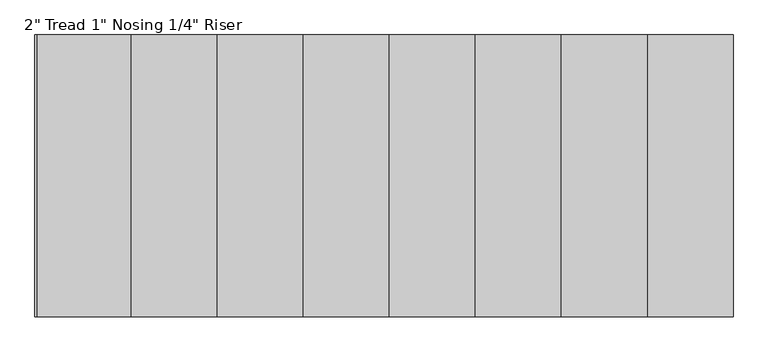
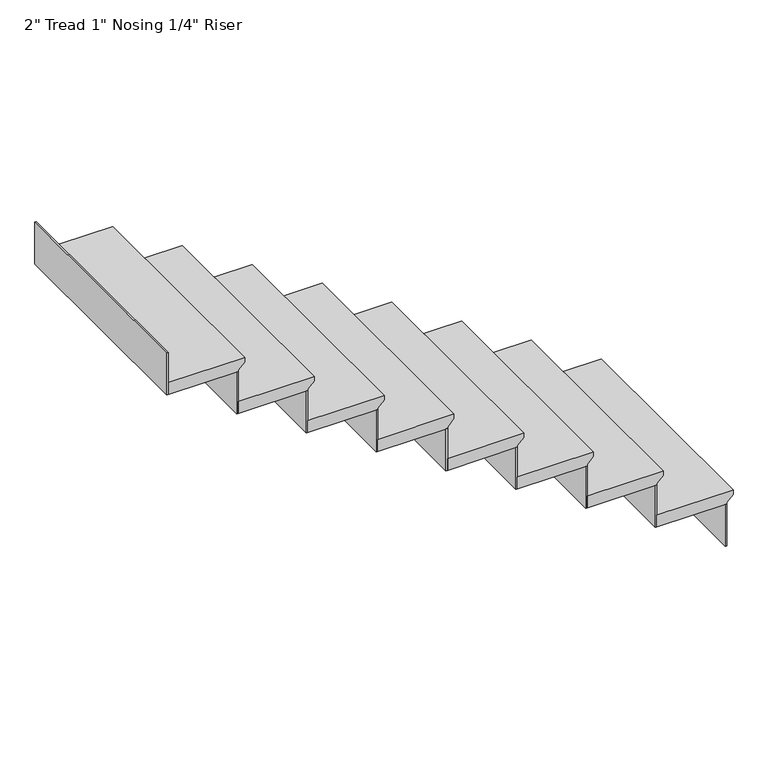
"""IFC4 building model written with IfcOpenShell, lengths in millimetres: stair flight geometry."""

from ifc_helpers import new_model, si_unit, frame, origin, place, context, project, spatial, polyline, outline, extrude, source, transform, mapped, element, save


def stair_flight_9d7122d5(model_context):
    return source(origin(), model_context, "Body", "SweptSolid", [
        extrude(outline(polyline([(1778.0, -2178.613859), (1778.0, -2483.413859), (1727.2, -2483.413859), (1727.2, -2204.013859), (1733.55, -2204.013859), (1758.95, -2178.613859), (1778.0, -2178.613859)])), frame((0.0, -712.1793133, 0.0), z_axis=(0.0, 1.0, 0.0), x_axis=(0.0, 0.0, 1.0)), (0.0, 0.0, 1.0), 914.4),
        extrude(outline(polyline([(-2210.363859, 202.2206867), (-2204.013859, 202.2206867), (-2204.013859, -712.1793133), (-2210.363859, -712.1793133), (-2210.363859, 202.2206867)])), frame((0.0, 0.0, 1549.4), z_axis=(0.0, 0.0, 1.0), x_axis=(1.0, 0.0, 0.0)), (0.0, 0.0, 1.0), 177.8),
        extrude(outline(polyline([(-2489.763859, 202.2206867), (-2483.413859, 202.2206867), (-2483.413859, -712.1793133), (-2489.763859, -712.1793133), (-2489.763859, 202.2206867)])), frame((0.0, 0.0, 1727.2), z_axis=(0.0, 0.0, 1.0), x_axis=(1.0, 0.0, 0.0)), (0.0, 0.0, 1.0), 177.8),
        extrude(outline(polyline([(1955.8, -2458.013859), (1955.8, -2762.813859), (1905.0, -2762.813859), (1905.0, -2483.413859), (1911.35, -2483.413859), (1936.75, -2458.013859), (1955.8, -2458.013859)])), frame((0.0, -712.1793133, 0.0), z_axis=(0.0, 1.0, 0.0), x_axis=(0.0, 0.0, 1.0)), (0.0, 0.0, 1.0), 914.4),
        extrude(outline(polyline([(-2769.163859, 202.2206867), (-2762.813859, 202.2206867), (-2762.813859, -712.1793133), (-2769.163859, -712.1793133), (-2769.163859, 202.2206867)])), frame((0.0, 0.0, 1905.0), z_axis=(0.0, 0.0, 1.0), x_axis=(1.0, 0.0, 0.0)), (0.0, 0.0, 1.0), 177.8),
        extrude(outline(polyline([(2133.6, -2737.413859), (2133.6, -3042.213859), (2082.8, -3042.213859), (2082.8, -2762.813859), (2089.15, -2762.813859), (2114.55, -2737.413859), (2133.6, -2737.413859)])), frame((0.0, -712.1793133, 0.0), z_axis=(0.0, 1.0, 0.0), x_axis=(0.0, 0.0, 1.0)), (0.0, 0.0, 1.0), 914.4),
        extrude(outline(polyline([(-3048.563859, 202.2206867), (-3042.213859, 202.2206867), (-3042.213859, -712.1793133), (-3048.563859, -712.1793133), (-3048.563859, 202.2206867)])), frame((0.0, 0.0, 2082.8), z_axis=(0.0, 0.0, 1.0), x_axis=(1.0, 0.0, 0.0)), (0.0, 0.0, 1.0), 177.8),
        extrude(outline(polyline([(2311.4, -3016.813859), (2311.4, -3321.613859), (2260.6, -3321.613859), (2260.6, -3042.213859), (2266.95, -3042.213859), (2292.35, -3016.813859), (2311.4, -3016.813859)])), frame((0.0, -712.1793133, 0.0), z_axis=(0.0, 1.0, 0.0), x_axis=(0.0, 0.0, 1.0)), (0.0, 0.0, 1.0), 914.4),
        extrude(outline(polyline([(-3327.963859, 202.2206867), (-3321.613859, 202.2206867), (-3321.613859, -712.1793133), (-3327.963859, -712.1793133), (-3327.963859, 202.2206867)])), frame((0.0, 0.0, 2260.6), z_axis=(0.0, 0.0, 1.0), x_axis=(1.0, 0.0, 0.0)), (0.0, 0.0, 1.0), 177.8),
        extrude(outline(polyline([(2489.2, -3296.213859), (2489.2, -3601.013859), (2438.4, -3601.013859), (2438.4, -3321.613859), (2444.75, -3321.613859), (2470.15, -3296.213859), (2489.2, -3296.213859)])), frame((0.0, -712.1793133, 0.0), z_axis=(0.0, 1.0, 0.0), x_axis=(0.0, 0.0, 1.0)), (0.0, 0.0, 1.0), 914.4),
        extrude(outline(polyline([(-3607.363859, 202.2206867), (-3601.013859, 202.2206867), (-3601.013859, -712.1793133), (-3607.363859, -712.1793133), (-3607.363859, 202.2206867)])), frame((0.0, 0.0, 2438.4), z_axis=(0.0, 0.0, 1.0), x_axis=(1.0, 0.0, 0.0)), (0.0, 0.0, 1.0), 177.8),
        extrude(outline(polyline([(2667.0, -3575.613859), (2667.0, -3880.413859), (2616.2, -3880.413859), (2616.2, -3601.013859), (2622.55, -3601.013859), (2647.95, -3575.613859), (2667.0, -3575.613859)])), frame((0.0, -712.1793133, 0.0), z_axis=(0.0, 1.0, 0.0), x_axis=(0.0, 0.0, 1.0)), (0.0, 0.0, 1.0), 914.4),
        extrude(outline(polyline([(-3886.763859, 202.2206867), (-3880.413859, 202.2206867), (-3880.413859, -712.1793133), (-3886.763859, -712.1793133), (-3886.763859, 202.2206867)])), frame((0.0, 0.0, 2616.2), z_axis=(0.0, 0.0, 1.0), x_axis=(1.0, 0.0, 0.0)), (0.0, 0.0, 1.0), 177.8),
        extrude(outline(polyline([(2844.8, -3855.013859), (2844.8, -4159.813859), (2794.0, -4159.813859), (2794.0, -3880.413859), (2800.35, -3880.413859), (2825.75, -3855.013859), (2844.8, -3855.013859)])), frame((0.0, -712.1793133, 0.0), z_axis=(0.0, 1.0, 0.0), x_axis=(0.0, 0.0, 1.0)), (0.0, 0.0, 1.0), 914.4),
        extrude(outline(polyline([(-4166.163859, 202.2206867), (-4159.813859, 202.2206867), (-4159.813859, -712.1793133), (-4166.163859, -712.1793133), (-4166.163859, 202.2206867)])), frame((0.0, 0.0, 2794.0), z_axis=(0.0, 0.0, 1.0), x_axis=(1.0, 0.0, 0.0)), (0.0, 0.0, 1.0), 177.8),
        extrude(outline(polyline([(-4445.563859, 202.2206867), (-4439.213859, 202.2206867), (-4439.213859, -712.1793133), (-4445.563859, -712.1793133), (-4445.563859, 202.2206867)])), frame((0.0, 0.0, 2971.8), z_axis=(0.0, 0.0, 1.0), x_axis=(1.0, 0.0, 0.0)), (0.0, 0.0, 1.0), 177.8),
        extrude(outline(polyline([(3022.6, -4134.413859), (3022.6, -4439.213859), (2971.8, -4439.213859), (2971.8, -4159.813859), (2978.15, -4159.813859), (3003.55, -4134.413859), (3022.6, -4134.413859)])), frame((0.0, -712.1793133, 0.0), z_axis=(0.0, 1.0, 0.0), x_axis=(0.0, 0.0, 1.0)), (0.0, 0.0, 1.0), 914.4),
    ])


if __name__ == "__main__":
    model = new_model("IFC4")
    model_context = context("Model", 3, world=origin())
    ifc_project = project(units=[si_unit("LENGTHUNIT", "METRE", prefix="MILLI")], contexts=[model_context])
    site = spatial("IfcSite", under=ifc_project)
    building = spatial("IfcBuilding", under=site)
    placement = place(None, origin())
    stair_flight_shape = stair_flight_9d7122d5(model_context)
    element("IfcStairFlight", 1, ObjectType="2\" Tread 1\" Nosing 1/4\" Riser", at=placement, inside=building, context=model_context, shape_type="MappedRepresentation", body=[
        mapped(stair_flight_shape, transform((0.0, 0.0, 0.0), x_axis=(1.0, 0.0, 0.0), y_axis=(0.0, 1.0, 0.0), z_axis=(0.0, 0.0, 1.0))),
    ])
    save(model, "model.ifc")
